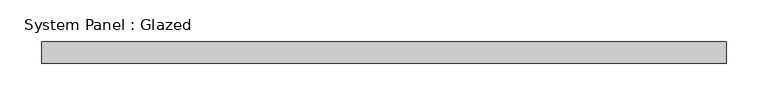
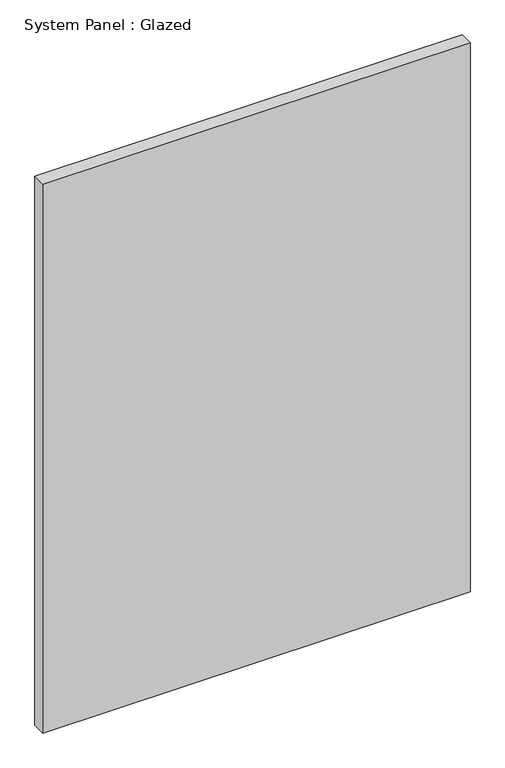
"""IFC4 building model written with IfcOpenShell, lengths in millimetres: plate geometry, System Panel : Glazed."""

from ifc_helpers import new_model, si_unit, origin, origin_with_axes, place, context, project, spatial, polyline, outline, extrude, source, transform, mapped, element, save


def system_panel_glazed_9025697b(model_context):
    return source(origin(), model_context, "Body", "SweptSolid", [
        extrude(outline(polyline([(409.575, 19.05), (-409.575, 19.05), (-409.575, 44.45), (409.575, 44.45), (409.575, 19.05)])), origin_with_axes(), (0.0, 0.0, 1.0), 1112.1384032),
    ])


if __name__ == "__main__":
    model = new_model("IFC4")
    model_context = context("Model", 3, world=origin())
    ifc_project = project(units=[si_unit("LENGTHUNIT", "METRE", prefix="MILLI")], contexts=[model_context])
    site = spatial("IfcSite", under=ifc_project)
    building = spatial("IfcBuilding", under=site)
    placement = place(None, origin())
    system_panel_glazed_shape = system_panel_glazed_9025697b(model_context)
    element("IfcPlate", 1, ObjectType="System Panel : Glazed", at=placement, inside=building, context=model_context, shape_type="MappedRepresentation", body=[
        mapped(system_panel_glazed_shape, transform((0.0, 0.0, 0.0), x_axis=(1.0, 0.0, 0.0), y_axis=(0.0, 1.0, 0.0), z_axis=(0.0, 0.0, 1.0))),
    ])
    save(model, "model.ifc")

# Revit data of these elements
# Type "System Panel : Glazed"
#   Construction Type Id = "GSP4R"
#   Analytic Construction = "1/8 in Pilkington single glazing"
#   Visual Light Transmittance = 0.9
#   Solar Heat Gain Coefficient = 0.86
#   Heat Transfer Coefficient (U) = 1.18115 BTU/(h·ft²·°F)
#   Define Thermal Properties by = 1
# Element 1 (IfcPlate, "System Panel : Glazed")
#   Materials on its faces: "Glass"
# Materials
#   "Glass": class "Glass", colour RGB 0 128 192, transparency 0.75, Description = "Soda Lime Glass", Cost = 0
